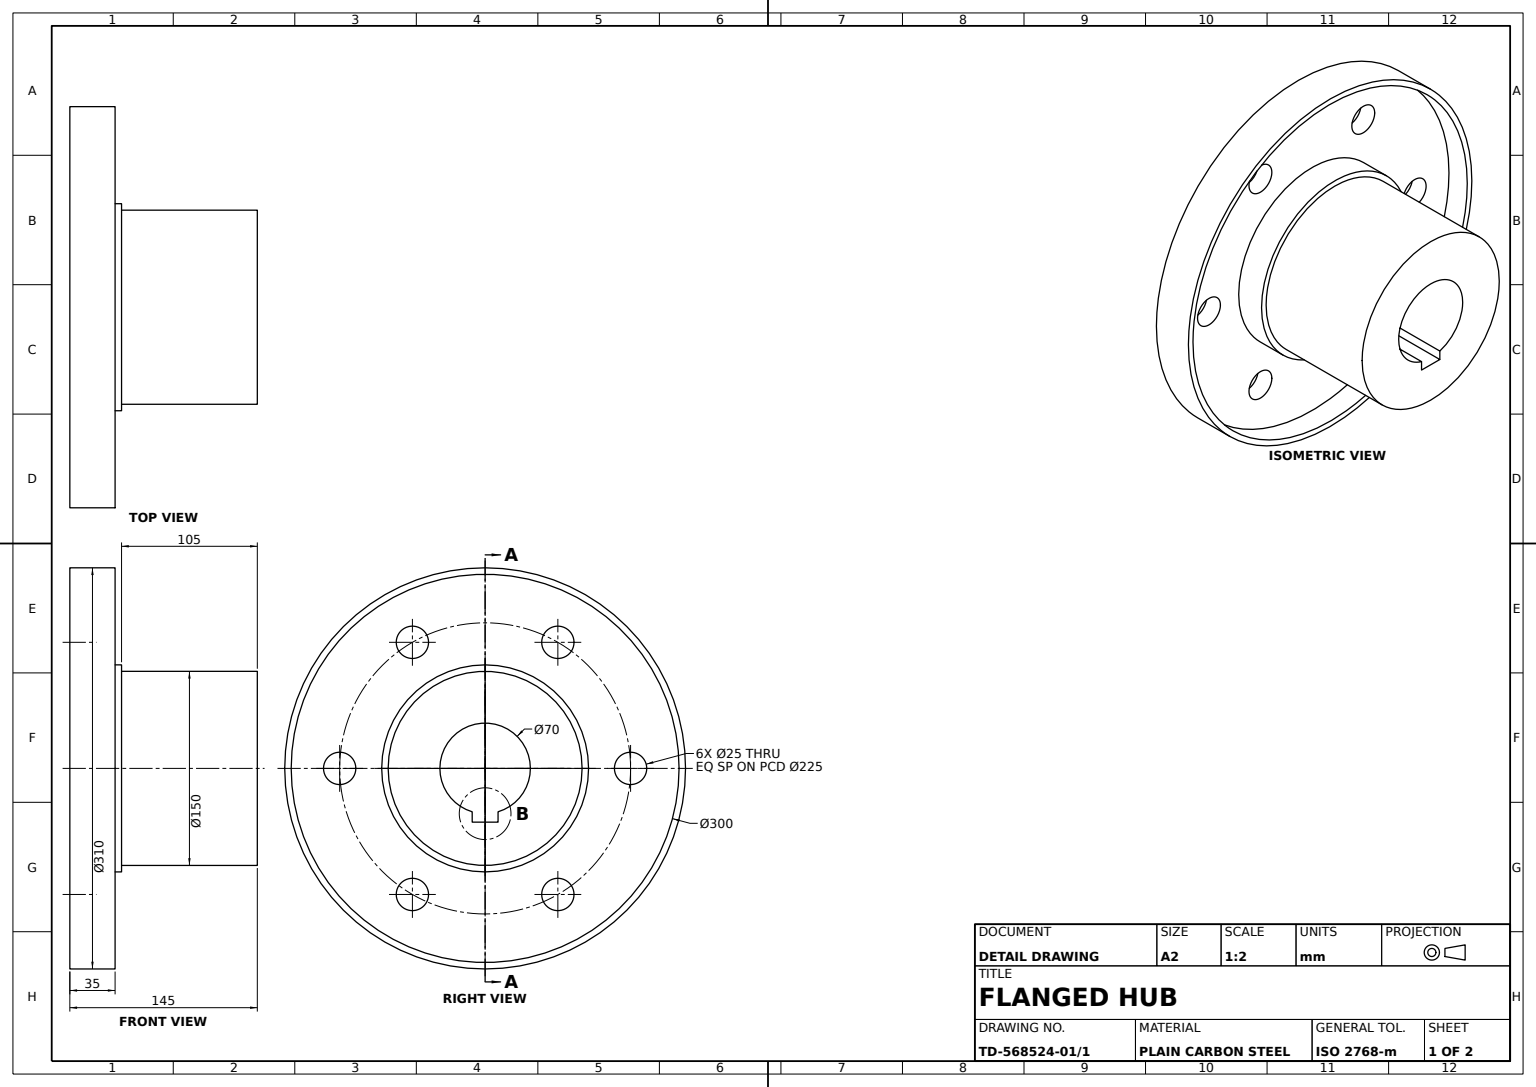
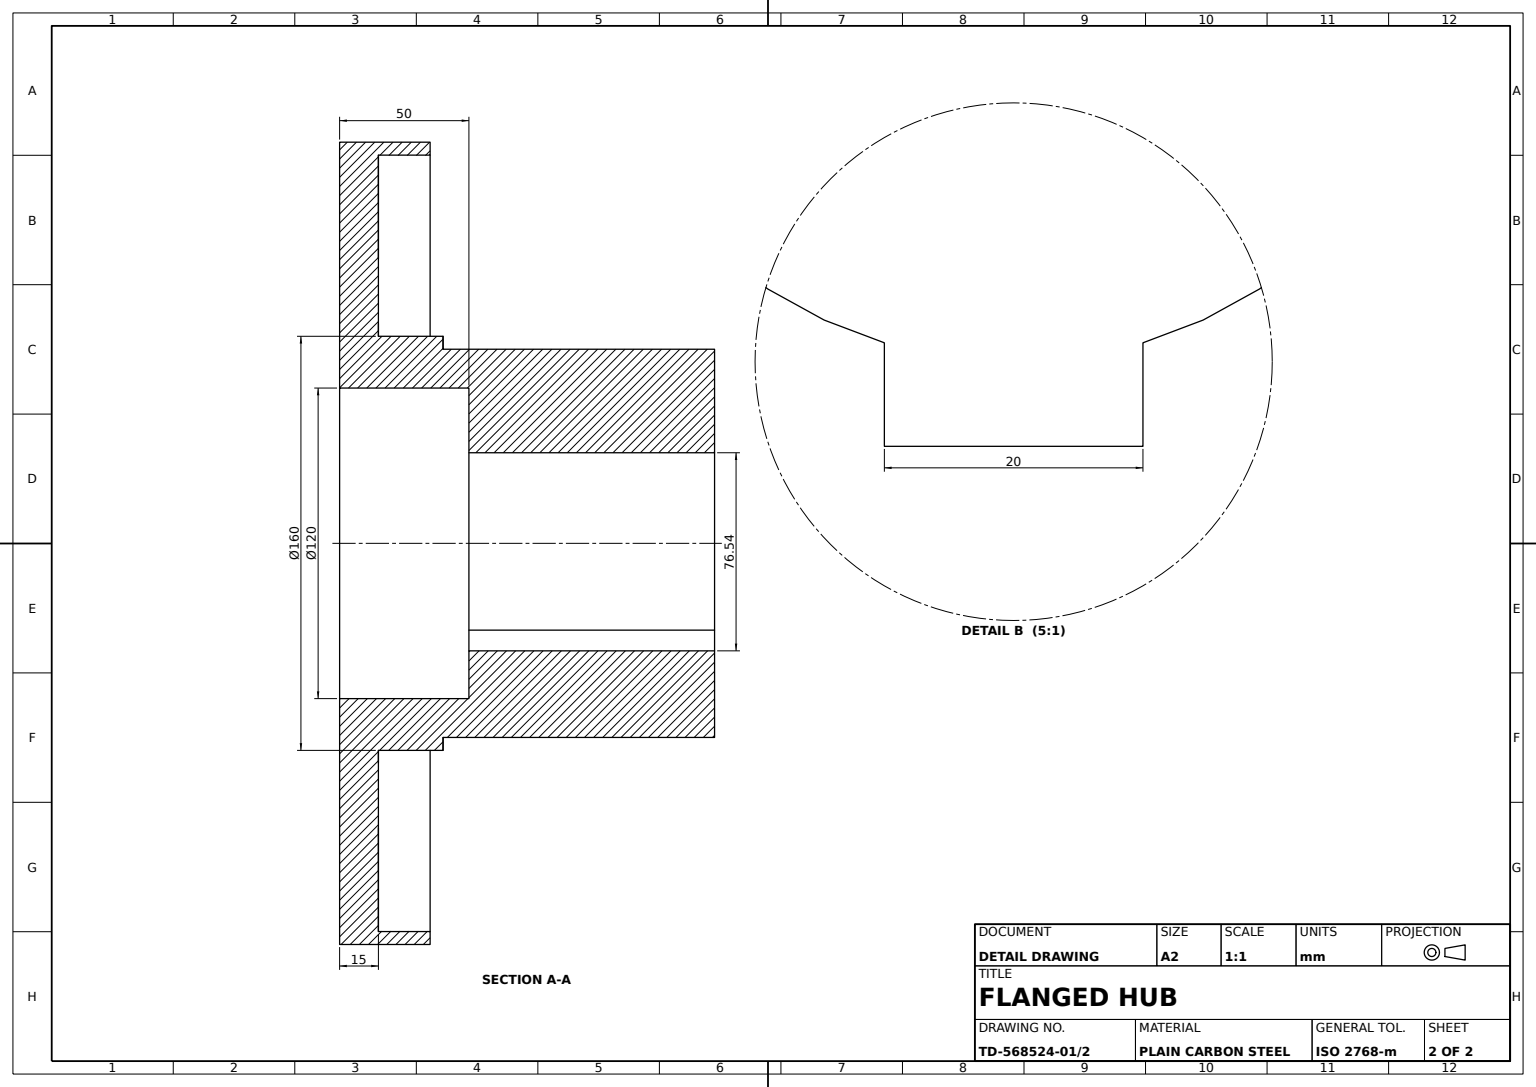
SolidWorks part; units mm, degrees
material "Plain Carbon Steel"
ref_plane "Front Plane" through (0, 0, 0) normal (0, 0, 1) x (1, 0, 0)
ref_plane "Top Plane" through (0, 0, 0) normal (0, 1, 0) x (1, 0, 0)
ref_plane "Right Plane" through (0, 0, 0) normal (1, 0, 0) x (0, 0, -1)
sketch "Flange Rim Sketch" plane through (0, 0, 0) normal (0, 1, 0) x (1, 0, 0)
  circle A0 centre (0, 0) radius 155
  circle A2 centre (0, 0) radius 150
  dimension "D1" = 310
  dimension "D2" = 300
extrude "Flange Rim Ø310" add sketch "Flange Rim Sketch" along normal blind 35
sketch "Flange Base Sketch" plane through (0, 0, 0) normal (0, 1, 0) x (1, 0, 0)
  circle A0 centre (0, 0) radius 150
  dimension "D1" = 300
extrude "Flange Base Disc" add sketch "Flange Base Sketch" along normal blind 15
sketch "Mounting Holes Sketch" plane through (0, 15, 0) normal (0, 1, 0) x (1, 0, 0)
  circle A1 centre (0, 112.5) radius 12.5
  circle A2 centre (97.4279, 56.25) radius 12.5
  circle A3 centre (97.4279, -56.25) radius 12.5
  circle A4 centre (0, -112.5) radius 12.5
  circle A5 centre (-97.4279, -56.25) radius 12.5
  circle A6 centre (-97.4279, 56.25) radius 12.5
  circle A7 centre (0, 0) radius 150 construction
  dimension "D1" = 97.4279
  dimension "D2" = 25
  dimension "D4" = 97.4279
  dimension "D5" = 56.25
  dimension "D3" = 6
extrude "Mounting Holes 6x" cut sketch "Mounting Holes Sketch" against normal blind 65
sketch "Hub Shoulder Sketch" plane through (0, 15, 0) normal (0, 1, 0) x (1, 0, 0)
  circle A0 centre (0, 0) radius 80
  dimension "D1" = 160
extrude "Hub Shoulder Ø160" add sketch "Hub Shoulder Sketch" along normal blind 25
sketch "Hub Sketch" plane through (0, 40, 0) normal (0, 1, 0) x (1, 0, 0)
  circle A0 centre (0, 0) radius 75
  dimension "D1" = 150
extrude "Hub Ø150" add sketch "Hub Sketch" along normal blind 105
sketch "Keyed Bore Sketch" plane through (0, 145, 0) normal (0, 1, 0) x (1, 0, 0)
  line L2 (41.541, 10) -> (33.541, 10)
  line L3 (41.541, -10) -> (33.541, -10)
  line L4 (41.541, 10) -> (41.541, -10)
  arc A0 (33.541, 10) -> (33.541, -10) centre (0, 0) ccw
  circle A1 centre (0, 0) radius 75 construction
  dimension "D1" = 8
  dimension "D3" = 35
  dimension "D2" = 8
  dimension "D4" = 33.541
extrude "Keyed Bore with Keyway 8x8" cut sketch "Keyed Bore Sketch" against normal blind 142
sketch "Recess Sketch" plane through (0, 0, 0) normal (0, -1, 0) x (1, 0, 0)
  circle A0 centre (0, 0) radius 60
  dimension "D1" = 120
extrude "Recess Ø120" cut sketch "Recess Sketch" against normal blind 50
